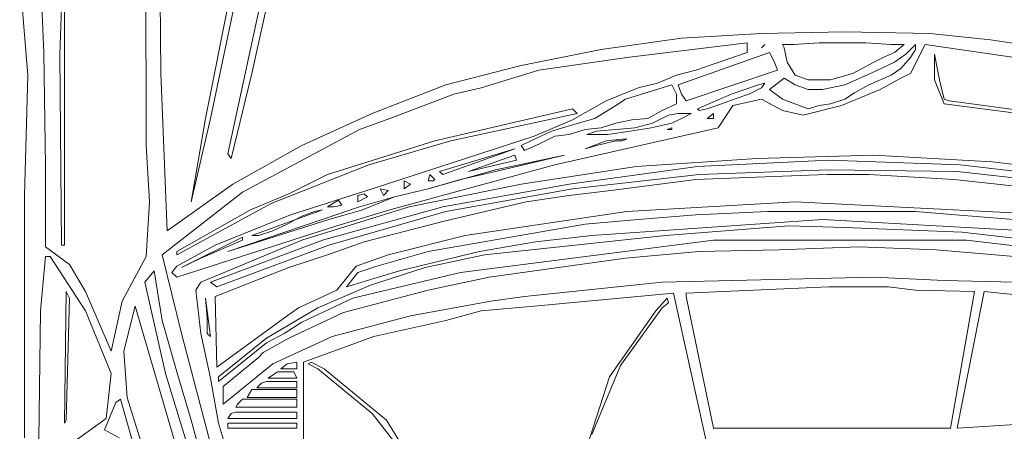
# Model space of a CAD drawing. Units: inches. Extents: x -9 to 646, y -802 to 47.
# Tile 7 of 17: x 432 to 465, y -575 to -561. Entities that reach past the tile are written whole.
import ezdxf

# ---------------------------------------------------------------- set-up
doc = ezdxf.new("R2010")
doc.units = ezdxf.units.IN
doc.header["$MEASUREMENT"] = 0
doc.layers.add('A-SITE-VEHI', color=8, linetype='Continuous', lineweight=9)

msp = doc.modelspace()

# ---------------------------------------------------------------- linework, layer by layer
at = {"layer": 'A-SITE-VEHI'}
for p, q in [((438.84, -565.895), (443.232, -545.569)), ((443.285, -546.437), (439.652, -563.186)), ((436.455, -547.63), (436.564, -563.186)), ((441.551, -549.146), (438.244, -564.703)), ((433.637, -549.797), (433.149, -562.536)), ((436.075, -564.756), (436.022, -552.237)), ((438.082, -564.703), (439.979, -555.164)), ((432.498, -559.771), (432.607, -562.48)), ((431.794, -559.933), (432.065, -563.239)), ((433.311, -568.984), (433.311, -560.964)), ((454.178, -561.994), (456.89, -561.83)), ((456.89, -561.83), (459.707, -561.776)), ((459.707, -561.776), (462.581, -561.83)), ((462.581, -561.83), (464.639, -562.047)), ((451.469, -562.371), (454.178, -561.994)), ((456.401, -562.156), (452.335, -562.642)), ((456.401, -562.48), (456.401, -562.156)), ((456.89, -562.318), (456.998, -562.209)), ((457.973, -562.209), (457.593, -562.209)), ((457.593, -562.209), (457.649, -562.318)), ((458.841, -562.156), (457.973, -562.209)), ((460.411, -562.156), (458.841, -562.156)), ((461.279, -562.209), (460.411, -562.156)), ((461.712, -562.209), (461.279, -562.209)), ((461.388, -562.48), (461.712, -562.209)), ((462.092, -562.209), (461.768, -562.536)), ((462.418, -562.209), (461.93, -563.186)), ((462.092, -562.371), (462.092, -562.209)), ((466.537, -562.806), (462.418, -562.209)), ((464.639, -562.047), (466.699, -562.371)), ((432.607, -562.48), (432.662, -566.328)), ((433.149, -562.536), (433.204, -568.984)), ((448.758, -562.915), (451.469, -562.371)), ((457.16, -562.48), (454.072, -563.564)), ((454.667, -563.077), (456.401, -562.48)), ((457.323, -562.806), (457.16, -562.48)), ((457.649, -562.318), (457.756, -562.806)), ((461.008, -562.642), (461.388, -562.48)), ((461.768, -562.536), (461.388, -562.806)), ((461.93, -562.642), (462.092, -562.371)), ((462.905, -563.402), (462.743, -562.536)), ((462.743, -562.536), (462.743, -563.402)), ((452.335, -562.642), (449.356, -563.077)), ((457.431, -563.077), (457.323, -562.806)), ((457.756, -562.806), (458.026, -563.239)), ((459.978, -563.186), (460.684, -562.806)), ((461.388, -562.806), (460.575, -563.186)), ((460.684, -562.806), (461.008, -562.642)), ((461.604, -563.022), (461.93, -562.642)), ((436.564, -563.186), (436.781, -568.497)), ((439.652, -563.186), (438.948, -566.057)), ((446.211, -563.564), (448.758, -562.915)), ((449.356, -563.077), (447.404, -563.673)), ((454.016, -563.239), (454.667, -563.077)), ((454.343, -564.108), (457.431, -563.077)), ((459.219, -563.402), (459.978, -563.186)), ((460.575, -563.186), (459.707, -563.564)), ((461.279, -563.239), (461.604, -563.022)), ((461.93, -563.186), (461.604, -563.348)), ((432.065, -563.239), (431.956, -567.305)), ((452.715, -563.673), (453.366, -563.51)), ((453.366, -563.51), (454.016, -563.239)), ((456.998, -563.51), (456.781, -563.564)), ((456.89, -563.673), (456.998, -563.51)), ((457.649, -563.348), (457.16, -563.728)), ((458.026, -563.564), (457.649, -563.348)), ((458.026, -563.239), (458.462, -563.402)), ((458.462, -563.402), (459.219, -563.402)), ((460.52, -563.564), (461.279, -563.239)), ((461.604, -563.348), (460.9, -563.728)), ((462.743, -563.402), (463.069, -564.214)), ((463.069, -564.052), (462.905, -563.402)), ((443.718, -564.541), (446.211, -563.564)), ((447.404, -563.673), (446.482, -563.89)), ((451.632, -564.108), (452.715, -563.673)), ((453.854, -563.564), (452.282, -564.052)), ((454.016, -563.89), (453.854, -563.564)), ((454.072, -563.564), (454.178, -563.89)), ((456.781, -563.564), (455.859, -563.89)), ((456.456, -563.89), (456.89, -563.673)), ((457.16, -563.728), (457.593, -564.052)), ((458.462, -563.728), (458.026, -563.564)), ((458.948, -563.728), (458.462, -563.728)), ((459.707, -563.564), (458.948, -563.728)), ((460.9, -563.728), (459.598, -564.27)), ((459.707, -564.052), (460.034, -563.835)), ((460.034, -563.835), (460.52, -563.564)), ((446.482, -563.89), (444.315, -564.703)), ((450.492, -564.756), (451.632, -564.108)), ((452.282, -564.052), (451.958, -564.27)), ((453.528, -564.432), (454.016, -564.214)), ((454.016, -564.214), (454.016, -563.89)), ((454.178, -563.89), (454.343, -564.108)), ((455.859, -563.89), (454.72, -564.379)), ((455.047, -564.379), (455.535, -564.214)), ((455.535, -564.214), (455.968, -564.052)), ((456.89, -564.052), (455.913, -564.27)), ((455.968, -564.052), (456.456, -563.89)), ((457.593, -564.432), (456.89, -564.052)), ((457.593, -564.052), (458.462, -564.379)), ((458.841, -564.27), (459.219, -564.214)), ((459.219, -564.214), (459.707, -564.052)), ((463.231, -564.108), (463.069, -564.052)), ((463.069, -564.214), (468.109, -564.865)), ((468.054, -564.756), (463.231, -564.108)), ((441.333, -565.624), (443.718, -564.541)), ((450.492, -564.379), (445.832, -565.462)), ((446.374, -565.462), (450.657, -564.541)), ((450.657, -564.541), (450.492, -564.379)), ((451.958, -564.27), (451.252, -564.703)), ((453.041, -564.703), (453.528, -564.432)), ((454.072, -564.541), (453.745, -564.594)), ((454.505, -564.541), (454.072, -564.541)), ((454.178, -564.703), (454.505, -564.541)), ((454.72, -564.379), (454.776, -564.432)), ((454.776, -564.432), (455.047, -564.379)), ((455.264, -564.541), (455.047, -564.703)), ((455.264, -564.703), (455.264, -564.541)), ((455.913, -564.27), (455.426, -565.027)), ((458.297, -564.594), (457.593, -564.432)), ((459.598, -564.27), (458.297, -564.594)), ((458.462, -564.379), (458.841, -564.27)), ((436.075, -565.624), (436.075, -564.756)), ((438.244, -564.703), (437.594, -567.521)), ((437.594, -567.521), (438.082, -564.703)), ((444.315, -564.703), (443.285, -565.082)), ((449.193, -565.3), (450.492, -564.756)), ((451.252, -564.703), (450.492, -564.92)), ((451.469, -565.027), (451.958, -564.865)), ((451.958, -564.865), (452.5, -564.756)), ((452.5, -564.756), (453.041, -564.703)), ((453.204, -564.865), (452.606, -565.027)), ((453.15, -565.027), (453.854, -564.865)), ((453.745, -564.594), (453.204, -564.865)), ((453.854, -564.865), (454.178, -564.703)), ((455.047, -564.703), (455.264, -564.703)), ((443.285, -565.082), (442.363, -565.571)), ((449.789, -565.136), (449.085, -565.462)), ((450.492, -564.92), (449.789, -565.136)), ((455.426, -565.027), (449.897, -566.275)), ((450.386, -565.245), (450.928, -565.082)), ((450.928, -565.082), (451.469, -565.027)), ((451.307, -565.136), (450.981, -565.245)), ((451.958, -565.082), (451.307, -565.136)), ((451.685, -565.245), (452.444, -565.136)), ((452.606, -565.027), (451.958, -565.082)), ((452.444, -565.136), (453.15, -565.027)), ((453.854, -565.027), (453.692, -565.082)), ((453.692, -565.082), (453.854, -565.082)), ((453.854, -565.082), (453.854, -565.027)), ((445.832, -565.462), (442.201, -566.599)), ((443.609, -566.275), (446.374, -565.462)), ((443.718, -567.088), (449.193, -565.3)), ((449.085, -565.462), (448.758, -565.624)), ((449.356, -565.571), (449.897, -565.3)), ((449.897, -565.3), (450.386, -565.245)), ((451.632, -565.462), (450.928, -565.733)), ((450.981, -565.245), (451.685, -565.245)), ((451.307, -565.624), (451.958, -565.462)), ((452.173, -565.407), (451.632, -565.462)), ((451.958, -565.462), (452.173, -565.462)), ((452.173, -565.462), (452.335, -565.407)), ((452.335, -565.407), (452.173, -565.407)), ((436.184, -567.521), (436.075, -565.624)), ((439.004, -566.925), (441.333, -565.624)), ((442.363, -565.571), (439.328, -567.196)), ((448.543, -565.733), (445.994, -566.492)), ((446.103, -566.599), (448.543, -565.733)), ((448.758, -565.624), (448.867, -565.786)), ((448.867, -565.786), (449.356, -565.571)), ((450.928, -565.733), (451.307, -565.624)), ((438.948, -566.057), (438.84, -565.895)), ((448.543, -565.948), (446.971, -566.492)), ((446.971, -566.492), (448.596, -566.113)), ((447.892, -566.437), (450.222, -565.948)), ((450.222, -565.948), (447.892, -566.492)), ((448.596, -566.113), (448.543, -565.948)), ((456.727, -566.057), (452.662, -566.328)), ((459.165, -566.113), (454.72, -566.328)), ((460.684, -565.948), (456.727, -566.057)), ((463.611, -566.275), (459.165, -566.113)), ((464.694, -566.166), (460.684, -565.948)), ((468.596, -566.655), (464.694, -566.166)), ((432.662, -566.328), (432.662, -569.039)), ((440.303, -567.576), (443.609, -566.275)), ((449.897, -566.275), (444.315, -567.791)), ((445.616, -567.088), (447.892, -566.437)), ((445.994, -566.492), (446.103, -566.599)), ((447.892, -566.492), (446.7, -566.763)), ((452.662, -566.328), (448.758, -566.925)), ((454.72, -566.328), (450.386, -566.925)), ((454.776, -566.599), (459.165, -566.437)), ((459.165, -566.437), (463.502, -566.492)), ((463.502, -566.492), (467.783, -566.979)), ((467.945, -566.763), (463.611, -566.275)), ((442.201, -566.599), (440.9, -567.25)), ((444.801, -566.817), (444.801, -567.088)), ((445.019, -566.925), (444.801, -566.817)), ((445.67, -566.599), (445.616, -566.817)), ((446.7, -566.763), (445.616, -567.088)), ((445.616, -566.817), (445.778, -566.817)), ((445.832, -566.763), (445.67, -566.599)), ((445.778, -566.817), (445.832, -566.763)), ((450.492, -567.088), (454.776, -566.599)), ((454.667, -566.763), (451.794, -567.141)), ((457.593, -566.655), (454.667, -566.763)), ((459.112, -566.599), (457.593, -566.655)), ((460.52, -566.599), (459.112, -566.599)), ((463.393, -566.763), (460.52, -566.599)), ((464.856, -566.925), (463.393, -566.763)), ((439.328, -567.196), (436.617, -569.31)), ((436.781, -568.497), (439.004, -566.925)), ((440.953, -567.956), (443.718, -567.088)), ((444.26, -567.141), (443.989, -567.088)), ((443.989, -567.088), (444.098, -567.305)), ((444.098, -567.305), (444.26, -567.141)), ((445.616, -567.088), (444.477, -567.358)), ((444.801, -567.088), (445.019, -566.925)), ((448.758, -566.925), (444.966, -567.685)), ((450.386, -566.925), (446.103, -567.685)), ((446.211, -567.847), (450.492, -567.088)), ((451.794, -567.141), (450.386, -567.305)), ((467.73, -567.25), (464.856, -566.925)), ((431.956, -567.305), (431.956, -575.49)), ((436.075, -569.364), (436.184, -567.521)), ((440.9, -567.25), (439.599, -567.791)), ((442.581, -567.467), (442.201, -567.685)), ((442.688, -567.629), (442.581, -567.467)), ((443.447, -567.25), (443.232, -567.305)), ((443.232, -567.305), (443.232, -567.521)), ((443.232, -567.521), (443.556, -567.358)), ((444.477, -567.358), (443.285, -567.685)), ((443.394, -567.791), (444.477, -567.358)), ((443.556, -567.358), (443.447, -567.25)), ((448.923, -567.521), (446.158, -568.171)), ((450.386, -567.305), (448.923, -567.521)), ((452.335, -567.847), (458.026, -567.521)), ((458.026, -567.521), (466.646, -567.956)), ((437.105, -569.31), (440.303, -567.576)), ((439.599, -567.791), (437.105, -569.201)), ((443.285, -567.685), (438.84, -569.201)), ((442.037, -567.791), (439.652, -568.66)), ((444.966, -567.685), (441.333, -568.822)), ((441.333, -568.009), (441.766, -567.847)), ((441.766, -567.847), (442.037, -567.791)), ((446.103, -567.685), (442.037, -568.822)), ((442.201, -567.685), (442.417, -567.685)), ((442.255, -568.118), (443.394, -567.791)), ((442.255, -568.984), (446.211, -567.847)), ((442.417, -567.685), (442.688, -567.629)), ((444.315, -567.791), (442.525, -568.335)), ((446.862, -568.66), (452.335, -567.847)), ((457.105, -567.847), (454.667, -567.956)), ((462.092, -567.847), (457.105, -567.847)), ((463.447, -567.956), (462.092, -567.847)), ((438.407, -568.984), (440.953, -567.956)), ((438.84, -569.201), (442.255, -568.118)), ((440.845, -568.28), (441.333, -568.009)), ((446.158, -568.171), (443.447, -568.877)), ((452.715, -568.118), (450.928, -568.28)), ((451.143, -568.66), (458.948, -568.118)), ((454.667, -567.956), (452.715, -568.118)), ((458.948, -568.118), (466.699, -568.551)), ((466.049, -568.171), (463.447, -567.956)), ((442.525, -568.335), (437.105, -570.07)), ((439.87, -568.66), (440.358, -568.497)), ((440.358, -568.497), (440.845, -568.28)), ((450.928, -568.28), (445.616, -569.201)), ((457.811, -568.335), (453.637, -568.66)), ((459.707, -568.389), (457.811, -568.335)), ((463.664, -568.551), (459.707, -568.389)), ((439.328, -568.713), (437.267, -569.743)), ((441.333, -568.822), (437.918, -570.232)), ((437.918, -569.419), (439.328, -568.822)), ((442.037, -568.822), (438.244, -570.232)), ((439.328, -568.822), (439.328, -568.713)), ((439.652, -568.66), (439.87, -568.66)), ((443.447, -568.877), (442.201, -569.31)), ((444.26, -569.31), (446.862, -568.66)), ((446.7, -569.905), (455.264, -568.822)), ((447.35, -569.201), (449.247, -568.877)), ((453.637, -568.66), (447.513, -569.31)), ((449.247, -568.877), (451.143, -568.66)), ((455.264, -568.822), (463.826, -568.822)), ((470.765, -569.364), (463.664, -568.551)), ((463.826, -568.822), (469.897, -569.528)), ((432.662, -569.039), (433.475, -569.634)), ((433.204, -568.984), (433.311, -568.984)), ((437.105, -569.69), (438.407, -568.984)), ((437.105, -569.201), (437.105, -569.31)), ((438.46, -570.394), (442.255, -568.984)), ((445.616, -569.201), (443.88, -569.69)), ((444.639, -569.852), (447.35, -569.201)), ((454.776, -569.201), (452.282, -569.419)), ((457.485, -569.148), (454.776, -569.201)), ((460.196, -569.039), (457.485, -569.148)), ((462.798, -569.148), (460.196, -569.039)), ((468.054, -569.581), (462.798, -569.148)), ((432.498, -571.206), (432.662, -569.364)), ((432.662, -569.364), (432.824, -569.364)), ((432.824, -569.364), (434.017, -571.206)), ((435.262, -570.882), (436.075, -569.364)), ((436.617, -569.31), (437.267, -571.966)), ((437.267, -569.743), (437.918, -569.419)), ((442.201, -569.31), (440.9, -569.743)), ((443.176, -569.69), (444.26, -569.31)), ((447.513, -569.31), (445.507, -569.743)), ((452.282, -569.419), (447.675, -570.07)), ((433.475, -569.634), (434.017, -570.556)), ((436.346, -569.852), (436.022, -570.232)), ((436.617, -571.533), (436.346, -569.852)), ((436.943, -569.905), (437.105, -569.69)), ((440.9, -569.743), (438.407, -570.72)), ((442.525, -570.503), (443.176, -569.69)), ((442.852, -570.394), (444.639, -569.852)), ((443.88, -569.69), (443.232, -569.905)), ((445.507, -569.743), (443.665, -570.34)), ((437.105, -570.07), (436.943, -569.905)), ((443.232, -569.905), (442.852, -570.394)), ((443.067, -570.773), (446.7, -569.905)), ((447.675, -570.07), (445.616, -570.503)), ((453.528, -570.232), (460.684, -570.07)), ((460.684, -570.07), (463.069, -570.176)), ((463.069, -570.176), (465.454, -570.232)), ((436.022, -570.232), (436.726, -573.32)), ((437.918, -570.232), (437.756, -570.503)), ((437.756, -570.503), (437.918, -571.966)), ((438.244, -570.232), (438.46, -570.394)), ((441.224, -571.098), (442.525, -570.503)), ((443.665, -570.34), (441.875, -571.098)), ((445.616, -570.503), (442.743, -571.262)), ((448.867, -570.72), (453.528, -570.232)), ((459.165, -570.394), (454.343, -570.611)), ((461.171, -570.394), (459.165, -570.394)), ((462.092, -570.503), (461.171, -570.394)), ((464.097, -570.556), (462.092, -570.503)), ((433.311, -575.001), (433.366, -570.556)), ((433.366, -570.556), (433.475, -570.773)), ((433.475, -570.773), (433.366, -574.892)), ((434.017, -570.556), (434.883, -572.561)), ((438.082, -570.773), (438.244, -572.075)), ((438.136, -571.424), (438.082, -570.773)), ((438.407, -570.72), (438.46, -573.105)), ((441.333, -571.586), (443.067, -570.773)), ((447.73, -570.882), (448.867, -570.72)), ((453.907, -570.611), (449.193, -571.044)), ((453.312, -571.206), (453.692, -570.773)), ((453.692, -570.773), (453.745, -570.936)), ((455.426, -577.439), (453.907, -570.611)), ((454.343, -570.611), (454.343, -570.72)), ((454.343, -570.72), (455.264, -575.163)), ((463.284, -575.163), (464.097, -570.556)), ((464.423, -570.556), (463.502, -575.163)), ((470.71, -571.206), (464.423, -570.556)), ((432.445, -575.543), (432.498, -571.206)), ((434.017, -571.206), (434.883, -573.32)), ((434.883, -572.561), (435.262, -570.882)), ((435.698, -571.044), (435.318, -572.561)), ((437.105, -575.867), (435.698, -571.044)), ((441.875, -571.098), (440.141, -572.128)), ((440.845, -571.369), (441.224, -571.098)), ((445.019, -571.369), (447.73, -570.882)), ((447.404, -571.206), (446.211, -571.533)), ((449.193, -571.044), (447.404, -571.206)), ((451.74, -573.429), (453.312, -571.206)), ((453.528, -571.098), (452.12, -573.049)), ((453.745, -570.936), (453.528, -571.098)), ((437.105, -573.267), (436.617, -571.533)), ((438.136, -571.966), (438.136, -571.424)), ((438.46, -573.105), (440.845, -571.369)), ((442.743, -571.262), (440.9, -572.128)), ((442.363, -572.075), (445.019, -571.369)), ((446.211, -571.533), (443.773, -572.075)), ((440.738, -571.966), (441.333, -571.586)), ((437.267, -571.966), (438.298, -575.867)), ((437.918, -571.966), (438.244, -573.482)), ((438.244, -572.075), (438.136, -571.966)), ((440.141, -572.128), (438.515, -573.429)), ((440.9, -572.128), (440.032, -572.616)), ((440.141, -572.29), (440.738, -571.966)), ((440.358, -572.996), (442.363, -572.075)), ((443.773, -572.075), (441.389, -572.941)), ((438.515, -573.591), (440.141, -572.29)), ((435.318, -572.561), (435.425, -574.133)), ((439.87, -572.779), (438.677, -573.755)), ((440.032, -572.616), (439.87, -572.779)), ((438.677, -574.351), (440.358, -572.996)), ((440.629, -573.158), (440.845, -572.996)), ((441.171, -573.158), (440.629, -573.158)), ((440.845, -572.996), (441.171, -572.941)), ((441.171, -572.941), (441.171, -573.158)), ((441.389, -572.941), (441.389, -576.085)), ((441.659, -572.941), (441.551, -572.996)), ((441.551, -572.996), (441.875, -573.158)), ((442.092, -573.158), (441.659, -572.941)), ((441.875, -573.158), (443.718, -574.675)), ((444.206, -574.892), (442.092, -573.158)), ((452.12, -573.049), (451.143, -575.381)), ((434.883, -573.32), (434.721, -574.839)), ((436.726, -573.32), (438.407, -578.796)), ((437.594, -574.892), (437.105, -573.267)), ((438.244, -573.482), (438.515, -575.001)), ((438.515, -573.429), (438.515, -573.591)), ((440.196, -573.482), (440.52, -573.267)), ((441.171, -573.482), (440.196, -573.482)), ((440.52, -573.267), (441.062, -573.267)), ((441.062, -573.267), (441.171, -573.482)), ((450.981, -575.814), (451.74, -573.429)), ((438.677, -573.755), (438.677, -574.351)), ((439.49, -574.133), (439.652, -573.862)), ((439.652, -573.862), (441.171, -573.862)), ((439.816, -573.809), (439.979, -573.647)), ((441.171, -573.809), (439.816, -573.809)), ((439.979, -573.647), (440.141, -573.591)), ((440.141, -573.591), (441.171, -573.591)), ((441.171, -573.591), (441.171, -573.809)), ((441.171, -573.862), (441.171, -574.133)), ((435.047, -574.297), (435.209, -574.189)), ((435.209, -574.189), (436.075, -577.224)), ((435.425, -574.133), (436.075, -576.194)), ((439.166, -574.351), (439.328, -574.189)), ((439.328, -574.189), (441.171, -574.189)), ((441.171, -574.133), (439.49, -574.133)), ((441.171, -574.189), (441.171, -574.459)), ((434.667, -575.219), (435.047, -574.297)), ((439.11, -574.459), (439.166, -574.351)), ((441.171, -574.459), (439.11, -574.459)), ((434.721, -574.839), (433.746, -575.543)), ((438.84, -574.839), (438.948, -574.675)), ((441.171, -574.839), (438.84, -574.839)), ((438.948, -574.675), (439.11, -574.622)), ((439.11, -574.622), (441.171, -574.622)), ((441.171, -574.622), (441.171, -574.839)), ((443.718, -574.675), (445.29, -576.682)), ((433.366, -574.892), (433.311, -575.001)), ((438.515, -578.254), (437.594, -574.892)), ((438.515, -575.001), (438.948, -576.411)), ((438.84, -575.163), (438.84, -575.001)), ((438.84, -575.001), (441.171, -575.001)), ((441.171, -575.163), (438.84, -575.163)), ((441.171, -575.001), (441.171, -575.163)), ((445.507, -577.006), (444.206, -574.892)), ((455.264, -575.163), (463.284, -575.163)), ((463.502, -575.163), (466.211, -575.001)), ((435.154, -575.49), (434.667, -575.219))]:
    msp.add_line(p, q, dxfattribs=at)

doc.saveas('drawing.dxf')
